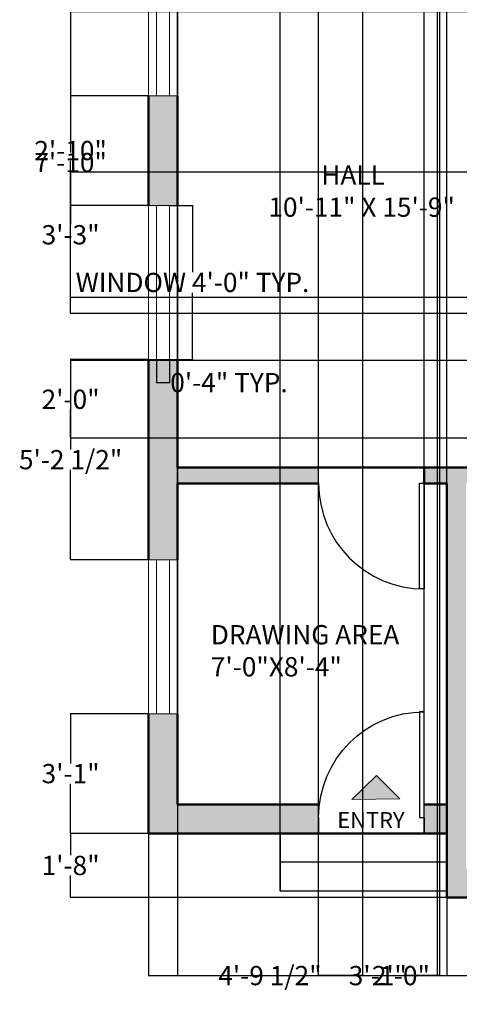
# Model space of a CAD drawing. Units: inches. Extents: x -19 to 356, y -14 to 509.
# Tile 1 of 3: x -19 to 118, y -14 to 293. Entities that reach past the tile are written whole.
import ezdxf

# ---------------------------------------------------------------- set-up
doc = ezdxf.new("R2010")
doc.units = ezdxf.units.IN
doc.header["$MEASUREMENT"] = 0
for name, color, linetype, lineweight in [('A-ANNO-DIMS', 7, 'Continuous', 18), ('A-ANNO-SYMB', 7, 'Continuous', 18), ('A-AREA-IDEN', 7, 'Continuous', 25), ('A-DOOR', 3, 'Continuous', 25), ('A-FLOR-STRS', 7, 'Continuous', 25), ('A-GLAZ', 5, 'Continuous', 18), ('A-WALL', 7, 'Continuous', 50), ('A-WALL-PATT', 4, 'Continuous', 13)]:
    doc.layers.add(name, color=color, linetype=linetype, lineweight=lineweight)
doc.styles.get("Standard").update_dxf_attribs({"font": 'arial.ttf'})
doc.dimstyles.get("Standard").update_dxf_attribs({"dimtxt": 6, "dimasz": 0.18, "dimexe": 0.18, "dimexo": 0.0625, "dimgap": 0.09, "dimtad": 0, "dimtih": 1, "dimtoh": 1, "dimzin": 0, "dimdsep": 46, "dimlunit": 3, "dimtxsty": 'Standard', "dimcen": 0.09, "dimadec": 0, "dimazin": 0, "dimtfac": 1, "dimtofl": 0, "dimtmove": 0, "dimatfit": 3, "dimfxl": 1, "dimtolj": 1, "dimtzin": 0, "dimarcsym": 0})

# ---------------------------------------------------------------- blocks, each defined once
blk = doc.blocks.new('*U2')
for p, q in [((0, 0), (0, -6)), ((40, 0), (40, -6))]:
    blk.add_line(p, q)
blk.add_lwpolyline([(0, 0), (0, 40), (1.75, 40), (1.75, 0)], close=True)
blk.add_arc((0, 0), 40, 0, 90)
blk = doc.blocks.new('GLAZ-UNIT-48IN')
for p, q in [((0, 48), (0, 0)), ((4, 48), (4, 0))]:
    blk.add_line(p, q)
blk = doc.blocks.new('*D13')
at = {"layer": 'A-ANNO-DIMS', "color": 0, "lineweight": -2, "transparency": 16777216}
for p, q in [((28.16, 235.01), (35.48, 235.01)), ((35.3, 234.83), (35.3, 214.2)), ((35.3, 187.19), (35.3, 207.82)), ((28.16, 187.01), (35.48, 187.01))]:
    blk.add_line(p, q, dxfattribs=at)
at = {"layer": 'A-ANNO-DIMS', "color": 0, "transparency": 16777216}
for points in [[(35.27, 234.83), (35.33, 234.83), (35.3, 235.01)], [(35.27, 187.19), (35.33, 187.19), (35.3, 187.01)]]:
    blk.add_solid(points, dxfattribs=at)
at = {"layer": 'Defpoints', "color": 0, "transparency": 16777216}
for p in [(28.1, 235.01), (35.3, 235.01), (28.1, 187.01)]:
    blk.add_point(p, dxfattribs=at)
at = {"layer": 'A-ANNO-DIMS', "color": 0, "transparency": 16777216, "insert": (35.3, 211.01), "char_height": 6, "attachment_point": 5}
blk.add_mtext('\\A1;WINDOW 4\'-0" TYP.', dxfattribs=at)
blk = doc.blocks.new('*D14')
at = {"layer": 'A-ANNO-DIMS', "color": 0, "lineweight": -2, "transparency": 16777216}
for p, q in [((24.1, 186.95), (24.1, 179.63)), ((28.1, 186.95), (28.1, 179.63)), ((24.28, 179.81), (27.92, 179.81)), ((28.1, 179.81), (28.28, 179.81))]:
    blk.add_line(p, q, dxfattribs=at)
at = {"layer": 'A-ANNO-DIMS', "color": 0, "transparency": 16777216}
for points in [[(24.28, 179.84), (24.28, 179.78), (24.1, 179.81)], [(27.92, 179.84), (27.92, 179.78), (28.1, 179.81)]]:
    blk.add_solid(points, dxfattribs=at)
at = {"layer": 'Defpoints', "color": 0, "transparency": 16777216}
for p in [(24.1, 187.01), (28.1, 187.01), (28.1, 179.81)]:
    blk.add_point(p, dxfattribs=at)
at = {"layer": 'A-ANNO-DIMS', "color": 0, "transparency": 16777216, "insert": (46.66, 179.81), "char_height": 6, "attachment_point": 5}
blk.add_mtext('\\A1;0\'-4" TYP.', dxfattribs=at)
blk = doc.blocks.new('*D19')
at = {"layer": 'A-ANNO-DIMS', "color": 0, "lineweight": -2, "transparency": 16777216}
for p, q in [((298.6, 201.31), (298.6, -5.12)), ((21.6, 39.31), (21.6, -5.12)), ((21.78, -4.94), (149.65, -4.94)), ((298.42, -4.94), (170.55, -4.94))]:
    blk.add_line(p, q, dxfattribs=at)
at = {"layer": 'A-ANNO-DIMS', "color": 0, "transparency": 16777216}
for points in [[(21.78, -4.91), (21.78, -4.97), (21.6, -4.94)], [(298.42, -4.91), (298.42, -4.97), (298.6, -4.94)]]:
    blk.add_solid(points, dxfattribs=at)
at = {"layer": 'Defpoints', "color": 0, "transparency": 16777216}
for p in [(298.6, 201.37), (21.6, 39.37), (298.6, -4.94)]:
    blk.add_point(p, dxfattribs=at)
at = {"layer": 'A-ANNO-DIMS', "color": 0, "transparency": 16777216, "insert": (160.1, -4.94), "char_height": 6, "attachment_point": 5}
blk.add_mtext('\\A1;23\'-1"', dxfattribs=at)
blk = doc.blocks.new('*D20')
at = {"layer": 'A-ANNO-DIMS', "color": 0, "lineweight": -2, "transparency": 16777216}
for p, q in [((21.54, 39.37), (-2.9, 39.37)), ((-2.72, 39.19), (-2.72, 32.53)), ((-2.72, 19.55), (-2.72, 26.22)), ((114.54, 19.37), (-2.9, 19.37))]:
    blk.add_line(p, q, dxfattribs=at)
at = {"layer": 'A-ANNO-DIMS', "color": 0, "transparency": 16777216}
for points in [[(-2.75, 39.19), (-2.69, 39.19), (-2.72, 39.37)], [(-2.75, 19.55), (-2.69, 19.55), (-2.72, 19.37)]]:
    blk.add_solid(points, dxfattribs=at)
at = {"layer": 'Defpoints', "color": 0, "transparency": 16777216}
for p in [(21.6, 39.37), (-2.72, 19.37), (114.6, 19.37)]:
    blk.add_point(p, dxfattribs=at)
at = {"layer": 'A-ANNO-DIMS', "color": 0, "transparency": 16777216, "insert": (-2.72, 29.37), "char_height": 6, "attachment_point": 5}
blk.add_mtext('\\A1;1\'-8"', dxfattribs=at)
blk = doc.blocks.new('*D21')
at = {"layer": 'A-ANNO-DIMS', "color": 0, "lineweight": -2, "transparency": 16777216}
for p, q in [((30.6, 48.44), (30.6, 499.87)), ((30.78, 499.69), (44.54, 499.69)), ((74.42, 499.69), (60.66, 499.69)), ((74.6, 39.44), (74.6, 499.87))]:
    blk.add_line(p, q, dxfattribs=at)
at = {"layer": 'A-ANNO-DIMS', "color": 0, "transparency": 16777216}
for points in [[(30.78, 499.72), (30.78, 499.66), (30.6, 499.69)], [(74.42, 499.72), (74.42, 499.66), (74.6, 499.69)]]:
    blk.add_solid(points, dxfattribs=at)
at = {"layer": 'Defpoints', "color": 0, "transparency": 16777216}
for p in [(74.6, 499.69), (30.6, 48.37), (74.6, 39.37)]:
    blk.add_point(p, dxfattribs=at)
at = {"layer": 'A-ANNO-DIMS', "color": 0, "transparency": 16777216, "insert": (52.6, 499.69), "char_height": 6, "attachment_point": 5}
blk.add_mtext('\\A1;3\'-8"', dxfattribs=at)
blk = doc.blocks.new('*D22')
at = {"layer": 'A-ANNO-DIMS', "color": 0, "lineweight": -2, "transparency": 16777216}
for p, q in [((74.6, 39.44), (74.6, 499.87)), ((74.78, 499.69), (82.95, 499.69)), ((107.35, 499.69), (99.18, 499.69)), ((107.53, 39.44), (107.53, 499.87))]:
    blk.add_line(p, q, dxfattribs=at)
at = {"layer": 'A-ANNO-DIMS', "color": 0, "transparency": 16777216}
for points in [[(74.78, 499.72), (74.78, 499.66), (74.6, 499.69)], [(107.35, 499.72), (107.35, 499.66), (107.53, 499.69)]]:
    blk.add_solid(points, dxfattribs=at)
at = {"layer": 'Defpoints', "color": 0, "transparency": 16777216}
for p in [(107.53, 499.69), (74.6, 39.37), (107.53, 39.37)]:
    blk.add_point(p, dxfattribs=at)
at = {"layer": 'A-ANNO-DIMS', "color": 0, "transparency": 16777216, "insert": (91.07, 499.69), "char_height": 6, "attachment_point": 5}
blk.add_mtext('\\A1;2\'-9"', dxfattribs=at)
blk = doc.blocks.new('*D23')
at = {"layer": 'A-ANNO-DIMS', "color": 0, "lineweight": -2, "transparency": 16777216}
for p, q in [((30.6, 466.31), (30.6, -5.12)), ((88.28, 466.31), (88.28, -5.12)), ((30.78, -4.94), (44.27, -4.94)), ((88.1, -4.94), (74.62, -4.94))]:
    blk.add_line(p, q, dxfattribs=at)
at = {"layer": 'A-ANNO-DIMS', "color": 0, "transparency": 16777216}
for points in [[(30.78, -4.91), (30.78, -4.97), (30.6, -4.94)], [(88.1, -4.91), (88.1, -4.97), (88.28, -4.94)]]:
    blk.add_solid(points, dxfattribs=at)
at = {"layer": 'Defpoints', "color": 0, "transparency": 16777216}
for p in [(30.6, 466.37), (88.28, 466.37), (88.28, -4.94)]:
    blk.add_point(p, dxfattribs=at)
at = {"layer": 'A-ANNO-DIMS', "color": 0, "transparency": 16777216, "insert": (59.44, -4.94), "char_height": 6, "attachment_point": 5}
blk.add_mtext('\\A1;4\'-9 1/2"', dxfattribs=at)
blk = doc.blocks.new('*D24')
at = {"layer": 'A-ANNO-DIMS', "color": 0, "lineweight": -2, "transparency": 16777216}
for p, q in [((88.28, 466.31), (88.28, -5.12)), ((112.28, 466.31), (112.28, -5.12)), ((88.46, -4.94), (92.17, -4.94)), ((112.1, -4.94), (108.4, -4.94))]:
    blk.add_line(p, q, dxfattribs=at)
at = {"layer": 'A-ANNO-DIMS', "color": 0, "transparency": 16777216}
for points in [[(88.46, -4.91), (88.46, -4.97), (88.28, -4.94)], [(112.1, -4.91), (112.1, -4.97), (112.28, -4.94)]]:
    blk.add_solid(points, dxfattribs=at)
at = {"layer": 'Defpoints', "color": 0, "transparency": 16777216}
for p in [(88.28, 466.37), (112.28, 466.37), (112.28, -4.94)]:
    blk.add_point(p, dxfattribs=at)
at = {"layer": 'A-ANNO-DIMS', "color": 0, "transparency": 16777216, "insert": (100.28, -4.94), "char_height": 6, "attachment_point": 5}
blk.add_mtext('\\A1;2\'-0"', dxfattribs=at)
blk = doc.blocks.new('*D25')
at = {"layer": 'A-ANNO-DIMS', "color": 0, "lineweight": -2, "transparency": 16777216}
for p, q in [((21.54, 76.59), (-2.9, 76.59)), ((-2.72, 76.41), (-2.72, 61.14)), ((-2.72, 39.55), (-2.72, 54.83)), ((21.54, 39.37), (-2.9, 39.37))]:
    blk.add_line(p, q, dxfattribs=at)
at = {"layer": 'A-ANNO-DIMS', "color": 0, "transparency": 16777216}
for points in [[(-2.75, 76.41), (-2.69, 76.41), (-2.72, 76.59)], [(-2.75, 39.55), (-2.69, 39.55), (-2.72, 39.37)]]:
    blk.add_solid(points, dxfattribs=at)
at = {"layer": 'Defpoints', "color": 0, "transparency": 16777216}
for p in [(-2.72, 76.59), (21.6, 76.59), (21.6, 39.37)]:
    blk.add_point(p, dxfattribs=at)
at = {"layer": 'A-ANNO-DIMS', "color": 0, "transparency": 16777216, "insert": (-2.72, 57.98), "char_height": 6, "attachment_point": 5}
blk.add_mtext('\\A1;3\'-1"', dxfattribs=at)
blk = doc.blocks.new('*D26')
at = {"layer": 'A-ANNO-DIMS', "color": 0, "lineweight": -2, "transparency": 16777216}
for p, q in [((21.54, 187.01), (-2.9, 187.01)), ((-2.72, 186.83), (-2.72, 158.99)), ((-2.72, 124.77), (-2.72, 152.61)), ((21.54, 124.59), (-2.9, 124.59))]:
    blk.add_line(p, q, dxfattribs=at)
at = {"layer": 'A-ANNO-DIMS', "color": 0, "transparency": 16777216}
for points in [[(-2.75, 186.83), (-2.69, 186.83), (-2.72, 187.01)], [(-2.75, 124.77), (-2.69, 124.77), (-2.72, 124.59)]]:
    blk.add_solid(points, dxfattribs=at)
at = {"layer": 'Defpoints', "color": 0, "transparency": 16777216}
for p in [(-2.72, 187.01), (21.6, 187.01), (21.6, 124.59)]:
    blk.add_point(p, dxfattribs=at)
at = {"layer": 'A-ANNO-DIMS', "color": 0, "transparency": 16777216, "insert": (-2.72, 155.8), "char_height": 6, "attachment_point": 5}
blk.add_mtext('\\A1;5\'-2 1/2"', dxfattribs=at)
blk = doc.blocks.new('*D27')
at = {"layer": 'A-ANNO-DIMS', "color": 0, "lineweight": -2, "transparency": 16777216}
for p, q in [((21.54, 269.19), (-2.9, 269.19)), ((-2.72, 269.01), (-2.72, 255.25)), ((-2.72, 235.19), (-2.72, 248.95)), ((21.54, 235.01), (-2.9, 235.01))]:
    blk.add_line(p, q, dxfattribs=at)
at = {"layer": 'A-ANNO-DIMS', "color": 0, "transparency": 16777216}
for points in [[(-2.75, 269.01), (-2.69, 269.01), (-2.72, 269.19)], [(-2.75, 235.19), (-2.69, 235.19), (-2.72, 235.01)]]:
    blk.add_solid(points, dxfattribs=at)
at = {"layer": 'Defpoints', "color": 0, "transparency": 16777216}
for p in [(-2.72, 269.19), (21.6, 269.19), (21.6, 235.01)]:
    blk.add_point(p, dxfattribs=at)
at = {"layer": 'A-ANNO-DIMS', "color": 0, "transparency": 16777216, "insert": (-2.72, 252.1), "char_height": 6, "attachment_point": 5}
blk.add_mtext('\\A1;2\'-10"', dxfattribs=at)
blk = doc.blocks.new('*D29')
at = {"layer": 'A-ANNO-DIMS', "color": 0, "lineweight": -2, "transparency": 16777216}
for p, q in [((114.6, 19.31), (114.6, -5.12)), ((163.02, 19.31), (163.02, -5.12)), ((114.78, -4.94), (123.64, -4.94)), ((162.84, -4.94), (153.99, -4.94))]:
    blk.add_line(p, q, dxfattribs=at)
at = {"layer": 'A-ANNO-DIMS', "color": 0, "transparency": 16777216}
for points in [[(114.78, -4.91), (114.78, -4.97), (114.6, -4.94)], [(162.84, -4.91), (162.84, -4.97), (163.02, -4.94)]]:
    blk.add_solid(points, dxfattribs=at)
at = {"layer": 'Defpoints', "color": 0, "transparency": 16777216}
for p in [(114.6, 19.37), (163.02, 19.37), (114.6, -4.94)]:
    blk.add_point(p, dxfattribs=at)
at = {"layer": 'A-ANNO-DIMS', "color": 0, "transparency": 16777216, "insert": (138.81, -4.94), "char_height": 6, "attachment_point": 5}
blk.add_mtext('\\A1;4\'-0 1/2"', dxfattribs=at)
blk = doc.blocks.new('*D30')
at = {"layer": 'A-ANNO-DIMS', "color": 0, "lineweight": -2, "transparency": 16777216}
for p, q in [((74.5, 343.31), (74.5, -5.12)), ((111.6, 343.31), (111.6, -5.12)), ((74.68, -4.94), (84.99, -4.94)), ((111.42, -4.94), (101.11, -4.94))]:
    blk.add_line(p, q, dxfattribs=at)
at = {"layer": 'A-ANNO-DIMS', "color": 0, "transparency": 16777216}
for points in [[(74.68, -4.91), (74.68, -4.97), (74.5, -4.94)], [(111.42, -4.91), (111.42, -4.97), (111.6, -4.94)]]:
    blk.add_solid(points, dxfattribs=at)
at = {"layer": 'Defpoints', "color": 0, "transparency": 16777216}
for p in [(74.5, 343.37), (111.6, 343.37), (111.6, -4.94)]:
    blk.add_point(p, dxfattribs=at)
at = {"layer": 'A-ANNO-DIMS', "color": 0, "transparency": 16777216, "insert": (93.05, -4.94), "char_height": 6, "attachment_point": 5}
blk.add_mtext('\\A1;3\'-1"', dxfattribs=at)
blk = doc.blocks.new('*D33')
at = {"layer": 'A-ANNO-DIMS', "color": 0, "lineweight": -2, "transparency": 16777216}
for p, q in [((74.6, 153.44), (74.6, 499.87)), ((74.78, 499.69), (82.95, 499.69)), ((107.35, 499.69), (99.18, 499.69)), ((107.53, 153.44), (107.53, 499.87))]:
    blk.add_line(p, q, dxfattribs=at)
at = {"layer": 'A-ANNO-DIMS', "color": 0, "transparency": 16777216}
for points in [[(74.78, 499.72), (74.78, 499.66), (74.6, 499.69)], [(107.35, 499.72), (107.35, 499.66), (107.53, 499.69)]]:
    blk.add_solid(points, dxfattribs=at)
at = {"layer": 'Defpoints', "color": 0, "transparency": 16777216}
for p in [(107.53, 499.69), (74.6, 153.37), (107.53, 153.37)]:
    blk.add_point(p, dxfattribs=at)
at = {"layer": 'A-ANNO-DIMS', "color": 0, "transparency": 16777216, "insert": (91.07, 499.69), "char_height": 6, "attachment_point": 5}
blk.add_mtext('\\A1;2\'-9"', dxfattribs=at)
blk = doc.blocks.new('*D35')
at = {"layer": 'A-ANNO-DIMS', "color": 0, "lineweight": -2, "transparency": 16777216}
for p, q in [((163.54, 186.72), (-2.9, 186.72)), ((-2.72, 186.54), (-2.72, 177.76)), ((-2.72, 162.67), (-2.72, 171.45)), ((163.54, 162.49), (-2.9, 162.49))]:
    blk.add_line(p, q, dxfattribs=at)
at = {"layer": 'A-ANNO-DIMS', "color": 0, "transparency": 16777216}
for points in [[(-2.75, 186.54), (-2.69, 186.54), (-2.72, 186.72)], [(-2.75, 162.67), (-2.69, 162.67), (-2.72, 162.49)]]:
    blk.add_solid(points, dxfattribs=at)
at = {"layer": 'Defpoints', "color": 0, "transparency": 16777216}
for p in [(-2.72, 186.72), (163.6, 186.72), (163.6, 162.49)]:
    blk.add_point(p, dxfattribs=at)
at = {"layer": 'A-ANNO-DIMS', "color": 0, "transparency": 16777216, "insert": (-2.72, 174.61), "char_height": 6, "attachment_point": 5}
blk.add_mtext('\\A1;2\'-0"', dxfattribs=at)
blk = doc.blocks.new('*D40')
at = {"layer": 'A-ANNO-DIMS', "color": 0, "lineweight": -2, "transparency": 16777216}
for p, q in [((168.54, 295.37), (-2.9, 295.37)), ((-2.72, 295.19), (-2.72, 251.53)), ((-2.72, 201.55), (-2.72, 245.22)), ((161.54, 201.37), (-2.9, 201.37))]:
    blk.add_line(p, q, dxfattribs=at)
at = {"layer": 'A-ANNO-DIMS', "color": 0, "transparency": 16777216}
for points in [[(-2.75, 295.19), (-2.69, 295.19), (-2.72, 295.37)], [(-2.75, 201.55), (-2.69, 201.55), (-2.72, 201.37)]]:
    blk.add_solid(points, dxfattribs=at)
at = {"layer": 'Defpoints', "color": 0, "transparency": 16777216}
for p in [(-2.72, 295.37), (168.6, 295.37), (161.6, 201.37)]:
    blk.add_point(p, dxfattribs=at)
at = {"layer": 'A-ANNO-DIMS', "color": 0, "transparency": 16777216, "insert": (-2.72, 248.37), "char_height": 6, "attachment_point": 5}
blk.add_mtext('\\A1;7\'-10"', dxfattribs=at)
blk = doc.blocks.new('*D44')
at = {"layer": 'A-ANNO-DIMS', "color": 0, "lineweight": -2, "transparency": 16777216}
for p, q in [((62.64, 21.44), (62.64, 499.87)), ((62.82, 499.69), (80.44, 499.69)), ((114.42, 499.69), (96.81, 499.69)), ((114.6, 21.44), (114.6, 499.87))]:
    blk.add_line(p, q, dxfattribs=at)
at = {"layer": 'A-ANNO-DIMS', "color": 0, "transparency": 16777216}
for points in [[(62.82, 499.72), (62.82, 499.66), (62.64, 499.69)], [(114.42, 499.72), (114.42, 499.66), (114.6, 499.69)]]:
    blk.add_solid(points, dxfattribs=at)
at = {"layer": 'Defpoints', "color": 0, "transparency": 16777216}
for p in [(114.6, 499.69), (62.64, 21.37), (114.6, 21.37)]:
    blk.add_point(p, dxfattribs=at)
at = {"layer": 'A-ANNO-DIMS', "color": 0, "transparency": 16777216, "insert": (88.62, 499.69), "char_height": 6, "attachment_point": 5}
blk.add_mtext('\\A1;4\'-4"', dxfattribs=at)
blk = doc.blocks.new('*D48')
at = {"layer": 'A-ANNO-DIMS', "color": 0, "lineweight": -2, "transparency": 16777216}
for p, q in [((171.54, 245.37), (-2.9, 245.37)), ((-2.72, 245.19), (-2.72, 229.03)), ((-2.72, 206.55), (-2.72, 222.72)), ((171.54, 206.37), (-2.9, 206.37))]:
    blk.add_line(p, q, dxfattribs=at)
at = {"layer": 'A-ANNO-DIMS', "color": 0, "transparency": 16777216}
for points in [[(-2.75, 245.19), (-2.69, 245.19), (-2.72, 245.37)], [(-2.75, 206.55), (-2.69, 206.55), (-2.72, 206.37)]]:
    blk.add_solid(points, dxfattribs=at)
at = {"layer": 'Defpoints', "color": 0, "transparency": 16777216}
for p in [(-2.72, 245.37), (171.6, 245.37), (171.6, 206.37)]:
    blk.add_point(p, dxfattribs=at)
at = {"layer": 'A-ANNO-DIMS', "color": 0, "transparency": 16777216, "insert": (-2.72, 225.87), "char_height": 6, "attachment_point": 5}
blk.add_mtext('\\A1;3\'-3"', dxfattribs=at)

msp = doc.modelspace()

# ---------------------------------------------------------------- hatches: boundary and pattern name
at = {"layer": 'A-ANNO-SYMB'}
h = msp.add_hatch(color=256, dxfattribs=at)
h.dxf.hatch_style = 1
h.paths.add_polyline_path([(92.644, 57.406), (84.933, 49.904), (99.906, 50.111)])
at = {"layer": 'A-WALL-PATT'}
h = msp.add_hatch(color=256, dxfattribs=at)
h.dxf.hatch_style = 1
h.paths.add_polyline_path([(74.504, 349.373), (30.6, 349.373), (30.6, 379.492), (21.6, 379.492), (21.6, 317.187), (30.6, 317.187), (30.6, 343.373), (74.504, 343.373)])
h.paths.add_polyline_path([(30.6, 269.187), (21.6, 269.187), (21.6, 235.01), (30.6, 235.01)])
h.paths.add_polyline_path([(30.6, 187.01), (21.6, 187.01), (21.6, 124.593), (30.6, 124.593), (30.6, 148.373), (74.604, 148.373), (74.604, 153.373), (30.6, 153.373)])
h.paths.add_polyline_path([(30.6, 76.593), (21.6, 76.593), (21.6, 39.373), (74.604, 39.373), (74.604, 44.312, -0.0309277), (74.855, 48.373), (30.6, 48.373)])
h.paths.add_polyline_path([(120.6, 148.373), (127.467, 148.373), (127.467, 148.483), (127.467, 153.373), (107.528, 153.373), (107.528, 148.373), (114.6, 148.373), (114.6, 19.373), (163.022, 19.373), (163.022, 28.373), (120.6, 28.373)])
h.paths.add_polyline_path([(114.6, 48.373), (107.528, 48.373), (107.528, 44.312), (107.528, 39.373), (114.6, 39.373)], flags=17)
h.paths.add_polyline_path([(261.6, 164.937), (252.6, 164.937), (252.6, 153.373), (168.6, 153.373), (168.6, 162.495), (167.233, 162.495), (163.6, 162.495), (163.6, 153.373), (160.071, 153.373), (160.071, 148.373), (252.6, 148.373), (252.6, 28.373), (211.022, 28.373), (211.022, 19.373), (261.6, 19.373)])
h.paths.add_polyline_path([(56.535, 228.167), (117.149, 228.167), (117.149, 250.555), (56.535, 250.555)], flags=9)
h.paths.add_polyline_path([(176.639, 359.092), (223.272, 359.092), (223.272, 381.481), (176.639, 381.481)], flags=9)

# ---------------------------------------------------------------- linework, layer by layer
at = {"layer": 'A-ANNO-SYMB'}
for p, q in [((84.933, 49.904), (92.644, 57.406)), ((92.644, 57.406), (99.906, 50.111)), ((84.933, 49.904), (99.906, 50.111))]:
    msp.add_line(p, q, dxfattribs=at)
at = {"layer": 'A-FLOR-STRS'}
msp.add_line((62.644, 39.373), (62.644, 21.373), dxfattribs=at)
for points in [[(114.6, 30.373), (62.644, 30.373)], [(114.6, 21.373), (62.644, 21.373)]]:
    msp.add_lwpolyline(points, dxfattribs=at)
at = {"layer": 'A-GLAZ'}
for points in [[(21.6, 317.187), (30.6, 317.187), (30.6, 269.187), (21.6, 269.187)], [(21.6, 235.01), (30.6, 235.01), (30.6, 187.01), (21.6, 187.01)], [(21.6, 124.593), (30.6, 124.593), (30.6, 76.593), (21.6, 76.593)]]:
    msp.add_lwpolyline(points, close=True, dxfattribs=at)
at = {"layer": 'A-WALL'}
msp.add_line((107.528, 148.373), (107.528, 153.373), dxfattribs=at)
for points in [[(21.6, 269.187), (21.6, 235.01)], [(30.6, 269.187), (30.6, 235.01)], [(21.6, 187.01), (21.6, 124.593)], [(30.6, 187.01), (30.6, 153.373)], [(163.6, 153.373), (30.6, 153.373)], [(30.6, 148.373), (30.6, 124.593)], [(74.604, 148.373), (30.6, 148.373)], [(114.6, 148.373), (107.528, 148.373)], [(114.6, 148.373), (114.6, 19.373)], [(21.6, 76.593), (21.6, 39.373)], [(30.6, 76.593), (30.6, 48.373)], [(74.855, 48.373), (30.6, 48.373)], [(114.6, 48.373), (107.528, 48.373)], [(114.6, 39.373), (21.6, 39.373)], [(114.6, 19.373), (163.022, 19.373)]]:
    msp.add_lwpolyline(points, dxfattribs=at)

# ---------------------------------------------------------------- block references
at = {"layer": 'A-DOOR', "xscale": 0.8231013004838734, "yscale": 0.8231013004838734, "zscale": 0.8231013004838734, "rotation": 180}
msp.add_blockref('*U2', (107.528, 148.435), dxfattribs=at)
at = {"layer": 'A-DOOR', "xscale": -0.8231013004838734, "yscale": 0.8231013004838734, "zscale": 0.8231013004838734}
msp.add_blockref('*U2', (107.528, 44.312), dxfattribs=at)
at = {"layer": 'A-GLAZ'}
for p in [(24.1, 269.188), (24.1, 187.01), (24.1, 76.593)]:
    msp.add_blockref('GLAZ-UNIT-48IN', p, dxfattribs=at)

# ---------------------------------------------------------------- texts
at = {"layer": 'A-AREA-IDEN', "attachment_point": 1}
for s, insert, char_height in [('         HALL\\P10\'-11" X 15\'-9"', (58.948, 247.467), 6), ('DRAWING AREA\\P7\'-0"X8\'-4"', (41.004, 104.259), 6), ('ENTRY', (80.428, 46), 5)]:
    msp.add_mtext_dynamic_manual_height_columns(s, width=102.62239, gutter_width=1, heights=[0], dxfattribs=dict(at, insert=insert, char_height=char_height))

# ---------------------------------------------------------------- dimensions: what is measured, and where the dimension line sits
at = {"layer": 'A-ANNO-DIMS'}
for base, p1, p2, picture, middle in [((74.604, 499.688), (30.6, 48.373), (74.604, 39.373), '*D21', (52.602, 499.688)), ((114.6, 499.688), (62.644, 21.373), (114.6, 21.373), '*D44', (88.622, 499.688)), ((107.528, 499.688), (74.604, 39.373), (107.528, 39.373), '*D22', (91.066, 499.688)), ((107.528, 499.688), (74.604, 153.373), (107.528, 153.373), '*D33', (91.066, 499.688)), ((88.282, -4.942), (30.6, 466.373), (88.282, 466.373), '*D23', (59.441, -4.942)), ((112.282, -4.942), (88.282, 466.373), (112.282, 466.373), '*D24', (100.282, -4.942)), ((111.6, -4.942), (74.504, 343.373), (111.6, 343.373), '*D30', (93.052, -4.942)), ((298.6, -4.942), (21.6, 39.373), (298.6, 201.373), '*D19', (160.1, -4.942)), ((114.6, -4.942), (163.022, 19.373), (114.6, 19.373), '*D29', (138.811, -4.942))]:
    dim = msp.add_linear_dim(base=base, p1=p1, p2=p2, dimstyle='Standard', override={"dimdec": 1, "dimlfac": 1, "dimrnd": 0, "dimzin": 1, "dimdsep": 46, "dimlunit": 4, "dimfrac": 2}, dxfattribs=at)
    dim.commit()
    dim.dimension.update_dxf_attribs({"geometry": picture, "text_midpoint": middle})
for base, p1, p2, picture, middle in [((-2.715, 295.373), (161.6, 201.373), (168.6, 295.373), '*D40', (-2.715, 248.373)), ((-2.715, 269.187), (21.6, 235.01), (21.6, 269.187), '*D27', (-2.715, 252.099)), ((-2.715, 245.373), (171.6, 206.373), (171.6, 245.373), '*D48', (-2.715, 225.873)), ((-2.715, 187.01), (21.6, 124.593), (21.6, 187.01), '*D26', (-2.715, 155.802)), ((-2.715, 186.717), (163.6, 162.495), (163.6, 186.717), '*D35', (-2.715, 174.606)), ((-2.715, 76.593), (21.6, 39.373), (21.6, 76.593), '*D25', (-2.715, 57.983)), ((-2.715, 19.373), (21.6, 39.373), (114.6, 19.373), '*D20', (-2.715, 29.373))]:
    dim = msp.add_linear_dim(base=base, p1=p1, p2=p2, angle=90, dimstyle='Standard', override={"dimdec": 1, "dimlfac": 1, "dimrnd": 0, "dimzin": 1, "dimdsep": 46, "dimlunit": 4, "dimfrac": 2}, dxfattribs=at)
    dim.commit()
    dim.dimension.update_dxf_attribs({"geometry": picture, "text_midpoint": middle})
dim = msp.add_linear_dim(base=(35.3, 235.01), p1=(28.1, 187.01), p2=(28.1, 235.01), angle=90, text='WINDOW <> TYP.', dimstyle='Standard', override={"dimdec": 1, "dimlfac": 1, "dimrnd": 0, "dimzin": 1, "dimdsep": 46, "dimlunit": 4, "dimfrac": 2}, dxfattribs=at)
dim.commit()
dim.dimension.update_dxf_attribs({"geometry": '*D13', "text_midpoint": (35.3, 211.01)})
dim = msp.add_linear_dim(base=(28.1, 179.81), p1=(24.1, 187.01), p2=(28.1, 187.01), text='<> TYP.', dimstyle='Standard', override={"dimdec": 1, "dimlfac": 1, "dimrnd": 0, "dimzin": 1, "dimdsep": 46, "dimlunit": 4, "dimfrac": 2}, dxfattribs=at)
dim.commit()
dim.dimension.update_dxf_attribs({"geometry": '*D14', "text_midpoint": (46.656, 179.81)})

doc.saveas('drawing.dxf')
